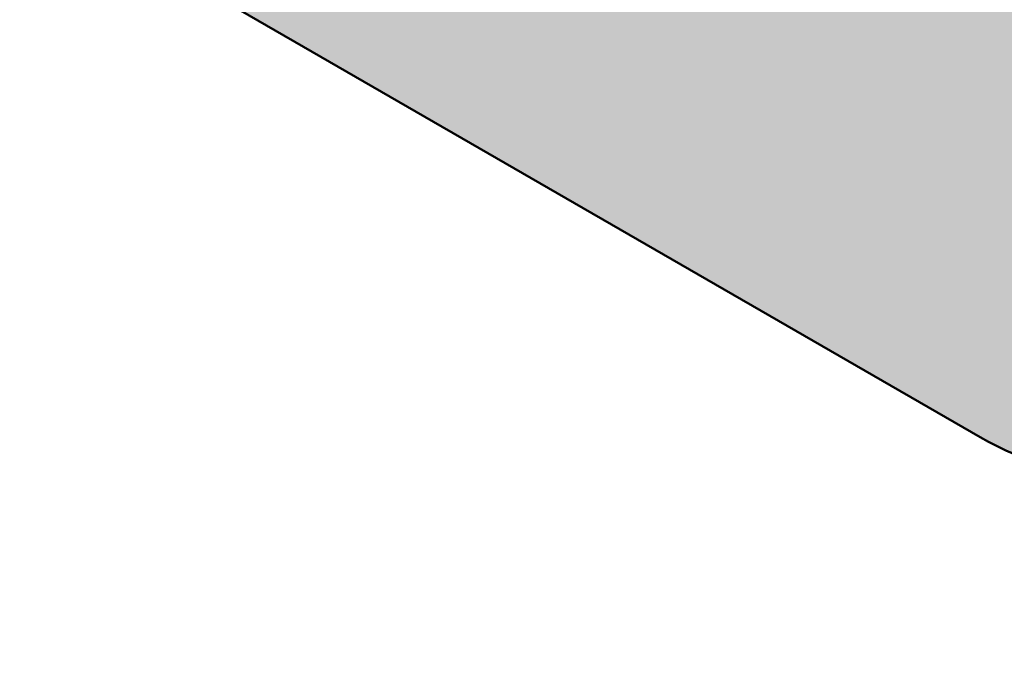
# Model space of a CAD drawing. Units: millimetres. Extents: x 0 to 2267, y 0 to 1823.
# Tile 22 of 256: x 1506 to 1590, y 1217 to 1271. Entities that reach past the tile are written whole.
import ezdxf

# ---------------------------------------------------------------- set-up
doc = ezdxf.new("R2010")
doc.units = ezdxf.units.MM
doc.header["$MEASUREMENT"] = 0
for name, color, linetype, lineweight in [('M-DIMS', 2, 'Continuous', 25), ('M-HATC', 252, 'Continuous', 18), ('M-OUTL', 7, 'Continuous', 50)]:
    doc.layers.add(name, color=color, linetype=linetype, lineweight=lineweight)
doc.styles.get("Standard").update_dxf_attribs({"font": 'arial.ttf'})
doc.dimstyles.get("Standard").update_dxf_attribs({"dimtxt": 7, "dimasz": 4, "dimexe": 0.18, "dimexo": 0.0625, "dimgap": 0.09, "dimtad": 0, "dimdec": 0, "dimzin": 0, "dimdsep": 46, "dimtxsty": 'Standard', "dimcen": 0.09, "dimadec": 0, "dimazin": 0, "dimtfac": 1, "dimtdec": 0, "dimtofl": 0, "dimtmove": 0, "dimatfit": 3, "dimfxl": 1, "dimtolj": 1, "dimtzin": 0, "dimarcsym": 0})

# ---------------------------------------------------------------- blocks, each defined once
blk = doc.blocks.new('*D19')
at = {"layer": 'Defpoints', "color": 0, "transparency": 16777216}
for p in [(1605.34, 1483.304), (1445.529, 1333.885)]:
    blk.add_point(p, dxfattribs=at)
at = {"layer": 'M-DIMS', "color": 0, "lineweight": -2, "transparency": 16777216}
for p, q in [((1605.25, 1483.304), (1605.43, 1483.304)), ((1605.34, 1483.214), (1605.34, 1483.394)), ((1366.324, 1259.831), (1442.607, 1331.153))]:
    blk.add_line(p, q, dxfattribs=at)
at = {"layer": 'M-DIMS', "color": 0, "transparency": 16777216}
blk.add_solid([(1442.152, 1331.64), (1443.063, 1330.666), (1445.529, 1333.885)], dxfattribs=at)
at = {"layer": 'M-DIMS', "color": 0, "transparency": 16777216, "insert": (1349.643, 1244.233), "char_height": 7, "attachment_point": 5, "rotation": 43.07533}
blk.add_mtext('\\A1;2X R218.8', dxfattribs=at)

msp = doc.modelspace()

# ---------------------------------------------------------------- hatches: boundary and pattern name
at = {"layer": 'M-HATC'}
h = msp.add_hatch(color=256, dxfattribs=at)
h.dxf.hatch_style = 1
h.paths.add_polyline_path([(2065.771, 1618.062, 0.236068), (2055.771, 1638.062), (1381.087, 1638.062, 0.236068), (1371.087, 1618.062), (1371.087, 1603.062), (2055.771, 1603.062), (2065.771, 1603.062)])
h.paths.add_polyline_path([(2062.772, 1550.296), (2062.772, 1560.296), (1374.086, 1560.296), (1374.086, 1550.296), (1374.086, 1540.296), (1384.086, 1540.296), (1389.086, 1540.296), (2062.772, 1540.296)])
h.paths.add_polyline_path([(1930.929, 1282.766), (1505.929, 1282.766), (1587.628, 1235.597, 0.131652), (1600.128, 1232.247), (1836.73, 1232.247, 0.131652), (1849.23, 1235.597)])
h.paths.add_polyline_path([(1930.929, 1117.417), (1905.929, 1117.417), (1505.929, 1117.417), (1505.929, 1077.417), (1930.929, 1077.417)])
h = msp.add_hatch(color=256, dxfattribs=at)
h.dxf.hatch_style = 1
h.paths.add_polyline_path([(2055.771, 1603.062), (1381.087, 1603.062), (1381.087, 1598.062), (2055.771, 1598.062)])
h.paths.add_polyline_path([(2055.771, 1598.062), (1381.087, 1598.062), (1381.087, 1593.062), (2055.771, 1593.062)])
h.paths.add_polyline_path([(2051.307, 1536.761), (1385.55, 1536.761), (1385.55, 1526.761), (1387.55, 1526.761), (1388.537, 1525.053), (1385.332, 1521.233), (1385.332, 1521.223), (2050.254, 1522.749), (2048.321, 1525.053), (2049.307, 1526.761), (2051.307, 1526.761)])
edge = h.paths.add_edge_path()
edge.add_arc((1847.535, 1379.149), 135, 222.60306, 222.89085, ccw=False)
edge.add_line((1748.166, 1287.766), (1683.092, 1287.766))
edge.add_arc((1583.724, 1379.149), 135, 317.10915, 317.39694, ccw=False)
edge.add_arc((1678.969, 1290.671), 5, 222.89085, 317.10915, ccw=False)
edge.add_arc((1774.213, 1379.149), 135, 222.60306, 222.89085, ccw=False)
edge.add_line((1674.845, 1287.766), (1609.771, 1287.766))
edge.add_arc((1510.403, 1379.149), 135, 317.10915, 317.39694, ccw=False)
edge.add_arc((1605.647, 1290.671), 5, 222.89085, 317.10915, ccw=False)
edge.add_arc((1700.892, 1379.149), 135, 222.60306, 222.89085, ccw=False)
edge.add_line((1601.524, 1287.766), (1536.45, 1287.766))
edge.add_arc((1437.081, 1379.149), 135, 317.10915, 317.39694, ccw=False)
edge.add_arc((1532.326, 1290.671), 5, 222.89085, 317.10915, ccw=False)
edge.add_arc((1627.571, 1379.149), 135, 222.60306, 222.89085, ccw=False)
edge.add_line((1528.203, 1287.766), (1505.929, 1287.766))
edge.add_spline(control_points=[(1505.929, 1287.766), (1504.262, 1287.766), (1504.262, 1282.766), (1505.929, 1282.766)], knot_values=[0, 0, 0, 0, 5, 5, 5, 5], degree=3, periodic=0)
edge.add_line((1505.929, 1282.766), (1930.929, 1282.766))
edge.add_spline(control_points=[(1930.929, 1282.766), (1932.596, 1282.766), (1932.596, 1287.766), (1930.929, 1287.766)], knot_values=[0, 0, 0, 0, 5, 5, 5, 5], degree=3, periodic=0)
edge.add_line((1930.929, 1287.766), (1903.056, 1287.766))
edge.add_arc((1803.688, 1379.149), 135, 317.10915, 317.39694, ccw=False)
edge.add_arc((1898.932, 1290.671), 5, 222.89085, 317.10915, ccw=False)
edge.add_arc((1994.177, 1379.149), 135, 222.60306, 222.89085, ccw=False)
edge.add_line((1894.809, 1287.766), (1829.735, 1287.766))
edge.add_arc((1730.366, 1379.149), 135, 317.10915, 317.39694, ccw=False)
edge.add_arc((1825.611, 1290.671), 5, 222.89085, 317.10915, ccw=False)
edge.add_arc((1920.856, 1379.149), 135, 222.60306, 222.89085, ccw=False)
edge.add_line((1821.487, 1287.766), (1756.413, 1287.766))
edge.add_arc((1657.045, 1379.149), 135, 317.10915, 317.39694, ccw=False)
edge.add_arc((1752.29, 1290.671), 5, 222.89085, 317.10915, ccw=False)
edge = h.paths.add_edge_path()
edge.add_spline(control_points=[(1843.429, 1227.247), (1845.096, 1227.247), (1845.096, 1232.247), (1843.429, 1232.247)], knot_values=[0, 0, 0, 0, 5, 5, 5, 5], degree=3, periodic=0)
edge.add_line((1843.429, 1232.247), (1593.429, 1232.247))
edge.add_spline(control_points=[(1593.429, 1232.247), (1591.762, 1232.247), (1591.762, 1227.247), (1593.429, 1227.247)], knot_values=[0, 0, 0, 0, 5, 5, 5, 5], degree=3, periodic=0)
edge.add_line((1593.429, 1227.247), (1843.429, 1227.247))
h.paths.add_polyline_path([(1905.929, 1127.417), (1530.929, 1127.417, 0.414214), (1520.929, 1117.417), (1530.929, 1117.417), (1915.929, 1117.417, 0.414214)])
edge = h.paths.add_edge_path()
edge.add_arc((1397.086, 1498.408), 12.73, 90.78215, 190.87871, ccw=False)
edge.add_line((1396.912, 1511.136), (1428.01, 1511.349))
edge.add_line((1428.01, 1511.349), (1433.01, 1511.349))
edge.add_line((1433.01, 1511.349), (1434.439, 1511.349))
edge.add_arc((1419.474, 1498.08), 20, 41.561, 74.08211)
edge.add_line((1424.959, 1517.314), (1399.935, 1517.256))
edge.add_spline(control_points=[(1399.931, 1517.256), (1399.884, 1517.213), (1399.833, 1517.169), (1399.777, 1517.124)], knot_values=[11.567499, 11.567499, 11.567499, 11.567499, 11.814249, 11.814249, 11.814249, 11.814249], degree=3, periodic=0)
edge.add_spline(control_points=[(1399.633, 1517.01), (1399.583, 1516.972), (1399.531, 1516.934), (1399.476, 1516.895)], knot_values=[11.167718, 11.167718, 11.167718, 11.167718, 11.365188, 11.365188, 11.365188, 11.365188], degree=3, periodic=0)
edge.add_spline(control_points=[(1399.34, 1516.8), (1399.151, 1516.672), (1398.938, 1516.538), (1398.704, 1516.399)], knot_values=[10.376405, 10.376405, 10.376405, 10.376405, 11.00994, 11.00994, 11.00994, 11.00994], degree=3, periodic=0)
edge.add_spline(control_points=[(1398.657, 1516.372), (1398.579, 1516.326), (1398.498, 1516.28), (1398.415, 1516.233)], knot_values=[10.125175, 10.125175, 10.125175, 10.125175, 10.334406, 10.334406, 10.334406, 10.334406], degree=3, periodic=0)
edge.add_spline(control_points=[(1398.264, 1516.149), (1398.196, 1516.111), (1398.126, 1516.073), (1398.055, 1516.035)], knot_values=[9.832246, 9.832246, 9.832246, 9.832246, 9.999658, 9.999658, 9.999658, 9.999658], degree=3, periodic=0)
edge.add_spline(control_points=[(1397.999, 1516.005), (1397.731, 1515.862), (1397.446, 1515.717), (1397.147, 1515.571)], knot_values=[9.161808, 9.161808, 9.161808, 9.161808, 9.787769, 9.787769, 9.787769, 9.787769], degree=3, periodic=0)
edge.add_spline(control_points=[(1397.147, 1515.571), (1396.842, 1515.423), (1396.522, 1515.274), (1396.191, 1515.126)], knot_values=[8.524455, 8.524455, 8.524455, 8.524455, 9.161808, 9.161808, 9.161808, 9.161808], degree=3, periodic=0)
edge.add_spline(control_points=[(1396.078, 1515.076), (1395.985, 1515.035), (1395.892, 1514.994), (1395.798, 1514.953)], knot_values=[8.275193, 8.275193, 8.275193, 8.275193, 8.451726, 8.451726, 8.451726, 8.451726], degree=3, periodic=0)
edge.add_spline(control_points=[(1395.602, 1514.869), (1395.5, 1514.826), (1395.397, 1514.782), (1395.293, 1514.739)], knot_values=[7.962917, 7.962917, 7.962917, 7.962917, 8.152764, 8.152764, 8.152764, 8.152764], degree=3, periodic=0)
edge.add_spline(control_points=[(1395.212, 1514.706), (1394.828, 1514.547), (1394.435, 1514.393), (1394.036, 1514.244)], knot_values=[7.21254, 7.21254, 7.21254, 7.21254, 7.913148, 7.913148, 7.913148, 7.913148], degree=3, periodic=0)
edge.add_spline(control_points=[(1394.036, 1514.244), (1393.708, 1514.121), (1393.375, 1514.003), (1393.043, 1513.889)], knot_values=[6.633733, 6.633733, 6.633733, 6.633733, 7.21254, 7.21254, 7.21254, 7.21254], degree=3, periodic=0)
edge.add_spline(control_points=[(1392.821, 1513.815), (1392.72, 1513.781), (1392.618, 1513.748), (1392.517, 1513.715)], knot_values=[6.328796, 6.328796, 6.328796, 6.328796, 6.505493, 6.505493, 6.505493, 6.505493], degree=3, periodic=0)
edge.add_spline(control_points=[(1392.517, 1513.715), (1392.319, 1513.652), (1392.121, 1513.59), (1391.924, 1513.531)], knot_values=[5.984605, 5.984605, 5.984605, 5.984605, 6.328796, 6.328796, 6.328796, 6.328796], degree=3, periodic=0)
edge.add_spline(control_points=[(1391.792, 1513.491), (1391.312, 1513.35), (1390.838, 1513.224), (1390.378, 1513.117)], knot_values=[5.066697, 5.066697, 5.066697, 5.066697, 5.907055, 5.907055, 5.907055, 5.907055], degree=3, periodic=0)
edge.add_spline(control_points=[(1390.378, 1513.117), (1390.18, 1513.071), (1389.984, 1513.028), (1389.791, 1512.99)], knot_values=[4.70367, 4.70367, 4.70367, 4.70367, 5.066695, 5.066695, 5.066695, 5.066695], degree=3, periodic=0)
edge.add_spline(control_points=[(1389.422, 1512.92), (1389.246, 1512.889), (1389.073, 1512.862), (1388.904, 1512.838)], knot_values=[4.130571, 4.130571, 4.130571, 4.130571, 4.469816, 4.469816, 4.469816, 4.469816], degree=3, periodic=0)
edge.add_spline(control_points=[(1388.904, 1512.838), (1388.591, 1512.795), (1388.291, 1512.764), (1388.007, 1512.749)], knot_values=[3.504031, 3.504031, 3.504031, 3.504031, 4.130571, 4.130571, 4.130571, 4.130571], degree=3, periodic=0)
edge.add_spline(control_points=[(1387.936, 1512.746), (1387.854, 1512.742), (1387.773, 1512.74), (1387.694, 1512.739)], knot_values=[3.268866, 3.268866, 3.268866, 3.268866, 3.451164, 3.451164, 3.451164, 3.451164], degree=3, periodic=0)
edge.add_spline(control_points=[(1387.335, 1512.744), (1387.208, 1512.75), (1387.085, 1512.76), (1386.967, 1512.774)], knot_values=[2.670686, 2.670686, 2.670686, 2.670686, 2.984, 2.984, 2.984, 2.984], degree=3, periodic=0)
edge.add_spline(control_points=[(1386.833, 1512.792), (1386.821, 1512.794), (1386.809, 1512.796), (1386.797, 1512.798)], knot_values=[2.516981, 2.516981, 2.516981, 2.516981, 2.549528, 2.549528, 2.549528, 2.549528], degree=3, periodic=0)
edge.add_spline(control_points=[(1386.453, 1512.873), (1386.426, 1512.881), (1386.399, 1512.889), (1386.373, 1512.897)], knot_values=[2.095869, 2.095869, 2.095869, 2.095869, 2.17941, 2.17941, 2.17941, 2.17941], degree=3, periodic=0)
edge.add_spline(control_points=[(1386.069, 1513.019), (1386.063, 1513.022), (1386.058, 1513.025), (1386.052, 1513.028)], knot_values=[1.72453, 1.72453, 1.72453, 1.72453, 1.745933, 1.745933, 1.745933, 1.745933], degree=3, periodic=0)
edge.add_arc((1399.474, 1498.08), 20, 131.82432, 180)
edge.add_arc((1630.334, 1505.548), 250.971, 181.70518, 236.42798)
edge.add_arc((1605.34, 1483.304), 218.782, 238.66083, 243.34961)
edge.add_arc((1647.091, 1510.359), 262.899, 183.12984, 237.85344, ccw=False)
h.paths.add_polyline_path([(1406.537, 1391.964, 0.149382), (1491.551, 1296.442, -0.129517)], flags=17)
edge = h.paths.add_edge_path()
edge.add_arc((2037.384, 1498.08), 20, 0, 48.26587)
edge.add_spline(control_points=[(2050.697, 1513.005), (2050.651, 1512.985), (2050.603, 1512.966), (2050.554, 1512.948)], knot_values=[1.835652, 1.835652, 1.835652, 1.835652, 2.000781, 2.000781, 2.000781, 2.000781], degree=3, periodic=0)
edge.add_spline(control_points=[(2050.462, 1512.917), (2050.479, 1512.922), (2050.496, 1512.928), (2050.513, 1512.934)], knot_values=[2.045477, 2.045477, 2.045477, 2.045477, 2.101389, 2.101389, 2.101389, 2.101389], degree=3, periodic=0)
edge.add_spline(control_points=[(2050.129, 1512.834), (2050.198, 1512.847), (2050.266, 1512.862), (2050.331, 1512.879)], knot_values=[2.237629, 2.237629, 2.237629, 2.237629, 2.435841, 2.435841, 2.435841, 2.435841], degree=3, periodic=0)
edge.add_spline(control_points=[(2050.095, 1512.828), (2050.106, 1512.83), (2050.118, 1512.832), (2050.129, 1512.834)], knot_values=[2.435841, 2.435841, 2.435841, 2.435841, 2.468321, 2.468321, 2.468321, 2.468321], degree=3, periodic=0)
edge.add_spline(control_points=[(2049.784, 1512.785), (2049.855, 1512.792), (2049.924, 1512.801), (2049.992, 1512.811)], knot_values=[2.563852, 2.563852, 2.563852, 2.563852, 2.748541, 2.748541, 2.748541, 2.748541], degree=3, periodic=0)
edge.add_spline(control_points=[(2049.405, 1512.762), (2049.536, 1512.765), (2049.663, 1512.773), (2049.784, 1512.785)], knot_values=[2.748541, 2.748541, 2.748541, 2.748541, 3.064882, 3.064882, 3.064882, 3.064882], degree=3, periodic=0)
edge.add_spline(control_points=[(2049.17, 1512.76), (2049.234, 1512.759), (2049.297, 1512.759), (2049.358, 1512.761)], knot_values=[3.102309, 3.102309, 3.102309, 3.102309, 3.2503, 3.2503, 3.2503, 3.2503], degree=3, periodic=0)
edge.add_spline(control_points=[(2048.857, 1512.769), (2048.964, 1512.764), (2049.068, 1512.761), (2049.17, 1512.76)], knot_values=[3.2503, 3.2503, 3.2503, 3.2503, 3.486069, 3.486069, 3.486069, 3.486069], degree=3, periodic=0)
edge.add_spline(control_points=[(2048.692, 1512.779), (2048.373, 1512.801), (2048.035, 1512.841), (2047.682, 1512.897)], knot_values=[3.606429, 3.606429, 3.606429, 3.606429, 4.2989, 4.2989, 4.2989, 4.2989], degree=3, periodic=0)
edge.add_spline(control_points=[(2047.682, 1512.897), (2047.546, 1512.919), (2047.408, 1512.942), (2047.268, 1512.969)], knot_values=[4.2989, 4.2989, 4.2989, 4.2989, 4.565769, 4.565769, 4.565769, 4.565769], degree=3, periodic=0)
edge.add_spline(control_points=[(2047.268, 1512.969), (2047.145, 1512.991), (2047.021, 1513.016), (2046.895, 1513.042)], knot_values=[4.565769, 4.565769, 4.565769, 4.565769, 4.799971, 4.799971, 4.799971, 4.799971], degree=3, periodic=0)
edge.add_spline(control_points=[(2046.895, 1513.042), (2046.529, 1513.119), (2046.151, 1513.209), (2045.768, 1513.311)], knot_values=[4.799971, 4.799971, 4.799971, 4.799971, 5.483718, 5.483718, 5.483718, 5.483718], degree=3, periodic=0)
edge.add_spline(control_points=[(2045.768, 1513.311), (2045.372, 1513.415), (2044.97, 1513.532), (2044.566, 1513.659)], knot_values=[5.483718, 5.483718, 5.483718, 5.483718, 6.187866, 6.187866, 6.187866, 6.187866], degree=3, periodic=0)
edge.add_spline(control_points=[(2044.566, 1513.659), (2044.415, 1513.706), (2044.263, 1513.755), (2044.112, 1513.805)], knot_values=[6.187866, 6.187866, 6.187866, 6.187866, 6.451551, 6.451551, 6.451551, 6.451551], degree=3, periodic=0)
edge.add_spline(control_points=[(2044.112, 1513.805), (2043.997, 1513.843), (2043.882, 1513.881), (2043.767, 1513.92)], knot_values=[6.451551, 6.451551, 6.451551, 6.451551, 6.651434, 6.651434, 6.651434, 6.651434], degree=3, periodic=0)
edge.add_spline(control_points=[(2043.767, 1513.92), (2043.372, 1514.055), (2042.977, 1514.198), (2042.589, 1514.346)], knot_values=[6.651434, 6.651434, 6.651434, 6.651434, 7.338879, 7.338879, 7.338879, 7.338879], degree=3, periodic=0)
edge.add_spline(control_points=[(2042.589, 1514.346), (2042.164, 1514.507), (2041.746, 1514.675), (2041.341, 1514.846)], knot_values=[7.338879, 7.338879, 7.338879, 7.338879, 8.089209, 8.089209, 8.089209, 8.089209], degree=3, periodic=0)
edge.add_spline(control_points=[(2041.341, 1514.846), (2041.103, 1514.946), (2040.869, 1515.048), (2040.64, 1515.15)], knot_values=[8.089209, 8.089209, 8.089209, 8.089209, 8.529587, 8.529587, 8.529587, 8.529587], degree=3, periodic=0)
edge.add_spline(control_points=[(2040.51, 1515.209), (2040.082, 1515.402), (2039.675, 1515.597), (2039.295, 1515.789)], knot_values=[8.613818, 8.613818, 8.613818, 8.613818, 9.44571, 9.44571, 9.44571, 9.44571], degree=3, periodic=0)
edge.add_spline(control_points=[(2039.295, 1515.789), (2039.062, 1515.907), (2038.839, 1516.025), (2038.629, 1516.14)], knot_values=[9.44571, 9.44571, 9.44571, 9.44571, 9.956404, 9.956404, 9.956404, 9.956404], degree=3, periodic=0)
edge.add_spline(control_points=[(2038.629, 1516.14), (2038.519, 1516.2), (2038.412, 1516.26), (2038.309, 1516.319)], knot_values=[9.956404, 9.956404, 9.956404, 9.956404, 10.223542, 10.223542, 10.223542, 10.223542], degree=3, periodic=0)
edge.add_spline(control_points=[(2038.309, 1516.319), (2038.214, 1516.374), (2038.122, 1516.428), (2038.033, 1516.481)], knot_values=[10.223542, 10.223542, 10.223542, 10.223542, 10.47051, 10.47051, 10.47051, 10.47051], degree=3, periodic=0)
edge.add_spline(control_points=[(2038.033, 1516.481), (2037.786, 1516.63), (2037.564, 1516.773), (2037.372, 1516.909)], knot_values=[10.47051, 10.47051, 10.47051, 10.47051, 11.15767, 11.15767, 11.15767, 11.15767], degree=3, periodic=0)
edge.add_spline(control_points=[(2037.372, 1516.909), (2037.279, 1516.975), (2037.193, 1517.04), (2037.114, 1517.102)], knot_values=[11.15767, 11.15767, 11.15767, 11.15767, 11.49227, 11.49227, 11.49227, 11.49227], degree=3, periodic=0)
edge.add_spline(control_points=[(2036.856, 1517.326), (2036.915, 1517.269), (2036.981, 1517.21), (2037.056, 1517.149)], knot_values=[11.577341, 11.577341, 11.577341, 11.577341, 11.91035, 11.91035, 11.91035, 11.91035], degree=3, periodic=0)
edge.add_spline(control_points=[(2036.807, 1517.375), (2036.823, 1517.359), (2036.839, 1517.342), (2036.856, 1517.326)], knot_values=[11.91035, 11.91035, 11.91035, 11.91035, 12.007402, 12.007402, 12.007402, 12.007402], degree=3, periodic=0)
edge.add_spline(control_points=[(2036.702, 1517.494), (2036.71, 1517.483), (2036.72, 1517.472), (2036.729, 1517.461)], knot_values=[12.184155, 12.184155, 12.184155, 12.184155, 12.255409, 12.255409, 12.255409, 12.255409], degree=3, periodic=0)
edge.add_spline(control_points=[(2036.616, 1517.621), (2036.62, 1517.613), (2036.624, 1517.606), (2036.629, 1517.598)], knot_values=[12.487913, 12.487913, 12.487913, 12.487913, 12.541035, 12.541035, 12.541035, 12.541035], degree=3, periodic=0)
edge.add_spline(control_points=[(2036.563, 1517.786), (2036.564, 1517.779), (2036.564, 1517.773), (2036.565, 1517.766)], knot_values=[12.911761, 12.911761, 12.911761, 12.911761, 12.968286, 12.968286, 12.968286, 12.968286], degree=3, periodic=0)
edge.add_spline(control_points=[(2036.617, 1517.93), (2036.612, 1517.926), (2036.609, 1517.921), (2036.605, 1517.916)], knot_values=[13.382527, 13.382527, 13.382527, 13.382527, 13.433791, 13.433791, 13.433791, 13.433791], degree=3, periodic=0)
edge.add_spline(control_points=[(2036.749, 1518.017), (2036.736, 1518.012), (2036.724, 1518.006), (2036.712, 1518)], knot_values=[13.726299, 13.726299, 13.726299, 13.726299, 13.809928, 13.809928, 13.809928, 13.809928], degree=3, periodic=0)
edge.add_spline(control_points=[(2036.86, 1518.053), (2036.839, 1518.047), (2036.818, 1518.042), (2036.799, 1518.035)], knot_values=[13.910887, 13.910887, 13.910887, 13.910887, 14.02153, 14.02153, 14.02153, 14.02153], degree=3, periodic=0)
edge.add_line((2036.964, 1518.08), (2032.384, 1518.08))
edge.add_line((2032.384, 1518.08), (2027.384, 1518.08))
edge.add_line((2027.384, 1518.08), (2022.384, 1518.08))
edge.add_line((2022.384, 1518.08), (2017.384, 1518.08))
edge.add_arc((2017.384, 1498.08), 20, 90, 138.439)
edge.add_line((2002.419, 1511.349), (2003.848, 1511.349))
edge.add_line((2003.848, 1511.349), (2008.848, 1511.349))
edge.add_line((2008.848, 1511.349), (2039.772, 1511.138))
edge.add_arc((2039.772, 1498.408), 12.73, -10.87871, 90, ccw=False)
edge.add_arc((1789.767, 1510.359), 262.899, 302.14656, 356.87016, ccw=False)
edge.add_arc((1831.518, 1483.304), 218.782, 296.65039, 301.33917)
edge.add_arc((1806.524, 1505.548), 250.971, 303.57202, 358.29482)
h.paths.add_polyline_path([(2030.321, 1391.964, -0.129517), (1945.307, 1296.442, 0.149382)], flags=17)
edge = h.paths.add_edge_path()
edge.add_spline(control_points=[(2037.246, 1518.082), (2037.29, 1518.081), (2037.336, 1518.08), (2037.384, 1518.08)], knot_values=[0.000012, 0.000012, 0.000012, 0.000012, 0.144754, 0.144754, 0.144754, 0.144754], degree=3, periodic=0)
edge.add_line((2037.336, 1518.08), (2037.01, 1518.08))
edge.add_spline(control_points=[(2037.01, 1518.08), (2036.982, 1518.077), (2036.956, 1518.073), (2036.931, 1518.068)], knot_values=[14.13465, 14.13465, 14.13465, 14.13465, 14.247197, 14.247197, 14.247197, 14.247197], degree=3, periodic=0)
edge.add_spline(control_points=[(2036.931, 1518.068), (2036.928, 1518.067), (2036.924, 1518.067), (2036.921, 1518.066)], knot_values=[14.118315, 14.118315, 14.118315, 14.118315, 14.13465, 14.13465, 14.13465, 14.13465], degree=3, periodic=0)
edge.add_spline(control_points=[(2036.921, 1518.066), (2036.912, 1518.064), (2036.903, 1518.063), (2036.895, 1518.061)], knot_values=[14.078086, 14.078086, 14.078086, 14.078086, 14.118315, 14.118315, 14.118315, 14.118315], degree=3, periodic=0)
edge.add_spline(control_points=[(2036.895, 1518.061), (2036.883, 1518.058), (2036.872, 1518.056), (2036.86, 1518.053)], knot_values=[14.02153, 14.02153, 14.02153, 14.02153, 14.078086, 14.078086, 14.078086, 14.078086], degree=3, periodic=0)
edge.add_spline(control_points=[(2036.86, 1518.053), (2036.839, 1518.047), (2036.818, 1518.042), (2036.799, 1518.035)], knot_values=[13.910887, 13.910887, 13.910887, 13.910887, 14.02153, 14.02153, 14.02153, 14.02153], degree=3, periodic=0)
edge.add_spline(control_points=[(2036.799, 1518.035), (2036.798, 1518.035), (2036.797, 1518.035), (2036.797, 1518.035)], knot_values=[13.906906, 13.906906, 13.906906, 13.906906, 13.910887, 13.910887, 13.910887, 13.910887], degree=3, periodic=0)
edge.add_spline(control_points=[(2036.797, 1518.035), (2036.788, 1518.032), (2036.78, 1518.029), (2036.772, 1518.026)], knot_values=[13.857826, 13.857826, 13.857826, 13.857826, 13.906906, 13.906906, 13.906906, 13.906906], degree=3, periodic=0)
edge.add_spline(control_points=[(2036.772, 1518.026), (2036.764, 1518.023), (2036.756, 1518.02), (2036.749, 1518.017)], knot_values=[13.809928, 13.809928, 13.809928, 13.809928, 13.857826, 13.857826, 13.857826, 13.857826], degree=3, periodic=0)
edge.add_spline(control_points=[(2036.749, 1518.017), (2036.736, 1518.012), (2036.724, 1518.006), (2036.712, 1518)], knot_values=[13.726299, 13.726299, 13.726299, 13.726299, 13.809928, 13.809928, 13.809928, 13.809928], degree=3, periodic=0)
edge.add_spline(control_points=[(2036.712, 1518), (2036.712, 1518), (2036.712, 1518), (2036.711, 1518)], knot_values=[13.723993, 13.723993, 13.723993, 13.723993, 13.726299, 13.726299, 13.726299, 13.726299], degree=3, periodic=0)
edge.add_spline(control_points=[(2036.711, 1518), (2036.706, 1517.997), (2036.701, 1517.994), (2036.696, 1517.992)], knot_values=[13.686536, 13.686536, 13.686536, 13.686536, 13.723993, 13.723993, 13.723993, 13.723993], degree=3, periodic=0)
edge.add_spline(control_points=[(2036.696, 1517.992), (2036.692, 1517.989), (2036.687, 1517.987), (2036.683, 1517.984)], knot_values=[13.651251, 13.651251, 13.651251, 13.651251, 13.686536, 13.686536, 13.686536, 13.686536], degree=3, periodic=0)
edge.add_spline(control_points=[(2036.683, 1517.984), (2036.676, 1517.98), (2036.67, 1517.976), (2036.664, 1517.971)], knot_values=[13.596804, 13.596804, 13.596804, 13.596804, 13.651251, 13.651251, 13.651251, 13.651251], degree=3, periodic=0)
edge.add_spline(control_points=[(2036.664, 1517.971), (2036.664, 1517.971), (2036.663, 1517.971), (2036.663, 1517.971)], knot_values=[13.593956, 13.593956, 13.593956, 13.593956, 13.596804, 13.596804, 13.596804, 13.596804], degree=3, periodic=0)
edge.add_spline(control_points=[(2036.663, 1517.971), (2036.66, 1517.969), (2036.658, 1517.967), (2036.655, 1517.965)], knot_values=[13.570322, 13.570322, 13.570322, 13.570322, 13.593956, 13.593956, 13.593956, 13.593956], degree=3, periodic=0)
edge.add_spline(control_points=[(2036.655, 1517.965), (2036.653, 1517.963), (2036.65, 1517.961), (2036.647, 1517.959)], knot_values=[13.545477, 13.545477, 13.545477, 13.545477, 13.570322, 13.570322, 13.570322, 13.570322], degree=3, periodic=0)
edge.add_spline(control_points=[(2036.647, 1517.959), (2036.647, 1517.959), (2036.647, 1517.959), (2036.647, 1517.959)], knot_values=[13.543931, 13.543931, 13.543931, 13.543931, 13.545477, 13.545477, 13.545477, 13.545477], degree=3, periodic=0)
edge.add_spline(control_points=[(2036.647, 1517.959), (2036.641, 1517.954), (2036.636, 1517.949), (2036.631, 1517.945)], knot_values=[13.488237, 13.488237, 13.488237, 13.488237, 13.543931, 13.543931, 13.543931, 13.543931], degree=3, periodic=0)
edge.add_spline(control_points=[(2036.631, 1517.945), (2036.628, 1517.942), (2036.626, 1517.94), (2036.623, 1517.937)], knot_values=[13.460307, 13.460307, 13.460307, 13.460307, 13.488237, 13.488237, 13.488237, 13.488237], degree=3, periodic=0)
edge.add_spline(control_points=[(2036.623, 1517.937), (2036.622, 1517.936), (2036.62, 1517.934), (2036.618, 1517.932)], knot_values=[13.439712, 13.439712, 13.439712, 13.439712, 13.460307, 13.460307, 13.460307, 13.460307], degree=3, periodic=0)
edge.add_spline(control_points=[(2036.618, 1517.932), (2036.618, 1517.931), (2036.617, 1517.931), (2036.617, 1517.93)], knot_values=[13.433791, 13.433791, 13.433791, 13.433791, 13.439712, 13.439712, 13.439712, 13.439712], degree=3, periodic=0)
edge.add_spline(control_points=[(2036.617, 1517.93), (2036.612, 1517.926), (2036.609, 1517.921), (2036.605, 1517.916)], knot_values=[13.382527, 13.382527, 13.382527, 13.382527, 13.433791, 13.433791, 13.433791, 13.433791], degree=3, periodic=0)
edge.add_spline(control_points=[(2036.605, 1517.916), (2036.603, 1517.913), (2036.6, 1517.91), (2036.598, 1517.907)], knot_values=[13.350017, 13.350017, 13.350017, 13.350017, 13.382527, 13.382527, 13.382527, 13.382527], degree=3, periodic=0)
edge.add_spline(control_points=[(2036.598, 1517.907), (2036.597, 1517.906), (2036.596, 1517.904), (2036.595, 1517.903)], knot_values=[13.333922, 13.333922, 13.333922, 13.333922, 13.350017, 13.350017, 13.350017, 13.350017], degree=3, periodic=0)
edge.add_spline(control_points=[(2036.595, 1517.903), (2036.595, 1517.902), (2036.594, 1517.901), (2036.593, 1517.9)], knot_values=[13.323828, 13.323828, 13.323828, 13.323828, 13.333922, 13.333922, 13.333922, 13.333922], degree=3, periodic=0)
edge.add_spline(control_points=[(2036.593, 1517.9), (2036.59, 1517.895), (2036.588, 1517.891), (2036.585, 1517.886)], knot_values=[13.277545, 13.277545, 13.277545, 13.277545, 13.323828, 13.323828, 13.323828, 13.323828], degree=3, periodic=0)
edge.add_spline(control_points=[(2036.585, 1517.886), (2036.584, 1517.883), (2036.582, 1517.879), (2036.58, 1517.875)], knot_values=[13.240119, 13.240119, 13.240119, 13.240119, 13.277545, 13.277545, 13.277545, 13.277545], degree=3, periodic=0)
edge.add_spline(control_points=[(2036.58, 1517.875), (2036.58, 1517.874), (2036.579, 1517.873), (2036.578, 1517.872)], knot_values=[13.228211, 13.228211, 13.228211, 13.228211, 13.240119, 13.240119, 13.240119, 13.240119], degree=3, periodic=0)
edge.add_spline(control_points=[(2036.578, 1517.872), (2036.578, 1517.87), (2036.577, 1517.869), (2036.577, 1517.868)], knot_values=[13.215717, 13.215717, 13.215717, 13.215717, 13.228211, 13.228211, 13.228211, 13.228211], degree=3, periodic=0)
edge.add_spline(control_points=[(2036.577, 1517.868), (2036.575, 1517.864), (2036.574, 1517.86), (2036.573, 1517.857)], knot_values=[13.179847, 13.179847, 13.179847, 13.179847, 13.215717, 13.215717, 13.215717, 13.215717], degree=3, periodic=0)
edge.add_spline(control_points=[(2036.573, 1517.857), (2036.571, 1517.851), (2036.57, 1517.846), (2036.569, 1517.841)], knot_values=[13.132017, 13.132017, 13.132017, 13.132017, 13.179847, 13.179847, 13.179847, 13.179847], degree=3, periodic=0)
edge.add_spline(control_points=[(2036.569, 1517.841), (2036.568, 1517.84), (2036.568, 1517.839), (2036.568, 1517.838)], knot_values=[13.122482, 13.122482, 13.122482, 13.122482, 13.132017, 13.132017, 13.132017, 13.132017], degree=3, periodic=0)
edge.add_spline(control_points=[(2036.568, 1517.838), (2036.568, 1517.836), (2036.567, 1517.835), (2036.567, 1517.833)], knot_values=[13.105592, 13.105592, 13.105592, 13.105592, 13.122482, 13.122482, 13.122482, 13.122482], degree=3, periodic=0)
edge.add_spline(control_points=[(2036.567, 1517.833), (2036.566, 1517.829), (2036.566, 1517.826), (2036.565, 1517.822)], knot_values=[13.074063, 13.074063, 13.074063, 13.074063, 13.105592, 13.105592, 13.105592, 13.105592], degree=3, periodic=0)
edge.add_spline(control_points=[(2036.565, 1517.822), (2036.565, 1517.822), (2036.565, 1517.822), (2036.565, 1517.822)], knot_values=[13.074043, 13.074043, 13.074043, 13.074043, 13.074063, 13.074063, 13.074063, 13.074063], degree=3, periodic=0)
edge.add_spline(control_points=[(2036.565, 1517.822), (2036.564, 1517.816), (2036.564, 1517.811), (2036.564, 1517.805)], knot_values=[13.021884, 13.021884, 13.021884, 13.021884, 13.074043, 13.074043, 13.074043, 13.074043], degree=3, periodic=0)
edge.add_spline(control_points=[(2036.564, 1517.805), (2036.564, 1517.804), (2036.564, 1517.803), (2036.564, 1517.803)], knot_values=[13.01674, 13.01674, 13.01674, 13.01674, 13.021884, 13.021884, 13.021884, 13.021884], degree=3, periodic=0)
edge.add_spline(control_points=[(2036.564, 1517.803), (2036.563, 1517.801), (2036.563, 1517.798), (2036.563, 1517.796)], knot_values=[12.996438, 12.996438, 12.996438, 12.996438, 13.01674, 13.01674, 13.01674, 13.01674], degree=3, periodic=0)
edge.add_spline(control_points=[(2036.563, 1517.796), (2036.563, 1517.793), (2036.563, 1517.789), (2036.563, 1517.786)], knot_values=[12.968286, 12.968286, 12.968286, 12.968286, 12.996438, 12.996438, 12.996438, 12.996438], degree=3, periodic=0)
edge.add_spline(control_points=[(2036.563, 1517.786), (2036.564, 1517.779), (2036.564, 1517.773), (2036.565, 1517.766)], knot_values=[12.911761, 12.911761, 12.911761, 12.911761, 12.968286, 12.968286, 12.968286, 12.968286], degree=3, periodic=0)
edge.add_spline(control_points=[(2036.565, 1517.766), (2036.565, 1517.766), (2036.565, 1517.766), (2036.565, 1517.766)], knot_values=[12.911017, 12.911017, 12.911017, 12.911017, 12.911761, 12.911761, 12.911761, 12.911761], degree=3, periodic=0)
edge.add_spline(control_points=[(2036.565, 1517.766), (2036.565, 1517.762), (2036.566, 1517.759), (2036.566, 1517.756)], knot_values=[12.88528, 12.88528, 12.88528, 12.88528, 12.911017, 12.911017, 12.911017, 12.911017], degree=3, periodic=0)
edge.add_spline(control_points=[(2036.566, 1517.756), (2036.567, 1517.753), (2036.567, 1517.751), (2036.568, 1517.748)], knot_values=[12.862519, 12.862519, 12.862519, 12.862519, 12.88528, 12.88528, 12.88528, 12.88528], degree=3, periodic=0)
edge.add_spline(control_points=[(2036.568, 1517.748), (2036.568, 1517.747), (2036.568, 1517.747), (2036.568, 1517.746)], knot_values=[12.858885, 12.858885, 12.858885, 12.858885, 12.862519, 12.862519, 12.862519, 12.862519], degree=3, periodic=0)
edge.add_spline(control_points=[(2036.568, 1517.746), (2036.569, 1517.74), (2036.571, 1517.733), (2036.572, 1517.726)], knot_values=[12.8053, 12.8053, 12.8053, 12.8053, 12.858885, 12.858885, 12.858885, 12.858885], degree=3, periodic=0)
edge.add_spline(control_points=[(2036.572, 1517.726), (2036.573, 1517.723), (2036.574, 1517.719), (2036.576, 1517.715)], knot_values=[12.775176, 12.775176, 12.775176, 12.775176, 12.8053, 12.8053, 12.8053, 12.8053], degree=3, periodic=0)
edge.add_spline(control_points=[(2036.576, 1517.715), (2036.576, 1517.713), (2036.577, 1517.71), (2036.578, 1517.708)], knot_values=[12.756759, 12.756759, 12.756759, 12.756759, 12.775176, 12.775176, 12.775176, 12.775176], degree=3, periodic=0)
edge.add_spline(control_points=[(2036.578, 1517.708), (2036.578, 1517.707), (2036.578, 1517.706), (2036.579, 1517.705)], knot_values=[12.748742, 12.748742, 12.748742, 12.748742, 12.756759, 12.756759, 12.756759, 12.756759], degree=3, periodic=0)
edge.add_spline(control_points=[(2036.579, 1517.705), (2036.581, 1517.698), (2036.583, 1517.692), (2036.586, 1517.685)], knot_values=[12.69959, 12.69959, 12.69959, 12.69959, 12.748742, 12.748742, 12.748742, 12.748742], degree=3, periodic=0)
edge.add_spline(control_points=[(2036.586, 1517.685), (2036.588, 1517.68), (2036.59, 1517.675), (2036.592, 1517.669)], knot_values=[12.659038, 12.659038, 12.659038, 12.659038, 12.69959, 12.69959, 12.69959, 12.69959], degree=3, periodic=0)
edge.add_spline(control_points=[(2036.592, 1517.669), (2036.594, 1517.665), (2036.596, 1517.66), (2036.598, 1517.656)], knot_values=[12.626806, 12.626806, 12.626806, 12.626806, 12.659038, 12.659038, 12.659038, 12.659038], degree=3, periodic=0)
edge.add_spline(control_points=[(2036.598, 1517.656), (2036.598, 1517.655), (2036.599, 1517.654), (2036.599, 1517.653)], knot_values=[12.619394, 12.619394, 12.619394, 12.619394, 12.626806, 12.626806, 12.626806, 12.626806], degree=3, periodic=0)
edge.add_spline(control_points=[(2036.599, 1517.653), (2036.604, 1517.642), (2036.61, 1517.632), (2036.616, 1517.621)], knot_values=[12.541039, 12.541039, 12.541039, 12.541039, 12.619394, 12.619394, 12.619394, 12.619394], degree=3, periodic=0)
edge.add_spline(control_points=[(2036.616, 1517.621), (2036.616, 1517.621), (2036.616, 1517.621), (2036.616, 1517.621)], knot_values=[12.541035, 12.541035, 12.541035, 12.541035, 12.541039, 12.541039, 12.541039, 12.541039], degree=3, periodic=0)
edge.add_spline(control_points=[(2036.616, 1517.621), (2036.62, 1517.613), (2036.624, 1517.606), (2036.629, 1517.598)], knot_values=[12.487913, 12.487913, 12.487913, 12.487913, 12.541035, 12.541035, 12.541035, 12.541035], degree=3, periodic=0)
edge.add_spline(control_points=[(2036.629, 1517.598), (2036.633, 1517.592), (2036.637, 1517.585), (2036.641, 1517.579)], knot_values=[12.443982, 12.443982, 12.443982, 12.443982, 12.487913, 12.487913, 12.487913, 12.487913], degree=3, periodic=0)
edge.add_spline(control_points=[(2036.641, 1517.579), (2036.641, 1517.578), (2036.642, 1517.576), (2036.643, 1517.575)], knot_values=[12.434996, 12.434996, 12.434996, 12.434996, 12.443982, 12.443982, 12.443982, 12.443982], degree=3, periodic=0)
edge.add_spline(control_points=[(2036.643, 1517.575), (2036.653, 1517.56), (2036.664, 1517.544), (2036.676, 1517.528)], knot_values=[12.329647, 12.329647, 12.329647, 12.329647, 12.434996, 12.434996, 12.434996, 12.434996], degree=3, periodic=0)
edge.add_spline(control_points=[(2036.676, 1517.528), (2036.684, 1517.517), (2036.693, 1517.505), (2036.702, 1517.494)], knot_values=[12.255409, 12.255409, 12.255409, 12.255409, 12.329647, 12.329647, 12.329647, 12.329647], degree=3, periodic=0)
edge.add_spline(control_points=[(2036.702, 1517.494), (2036.71, 1517.483), (2036.72, 1517.472), (2036.729, 1517.461)], knot_values=[12.184155, 12.184155, 12.184155, 12.184155, 12.255409, 12.255409, 12.255409, 12.255409], degree=3, periodic=0)
edge.add_spline(control_points=[(2036.729, 1517.461), (2036.744, 1517.444), (2036.759, 1517.426), (2036.775, 1517.409)], knot_values=[12.075961, 12.075961, 12.075961, 12.075961, 12.184155, 12.184155, 12.184155, 12.184155], degree=3, periodic=0)
edge.add_spline(control_points=[(2036.775, 1517.409), (2036.776, 1517.407), (2036.777, 1517.406), (2036.778, 1517.405)], knot_values=[12.069502, 12.069502, 12.069502, 12.069502, 12.075961, 12.075961, 12.075961, 12.075961], degree=3, periodic=0)
edge.add_spline(control_points=[(2036.778, 1517.405), (2036.788, 1517.395), (2036.797, 1517.385), (2036.807, 1517.375)], knot_values=[12.007402, 12.007402, 12.007402, 12.007402, 12.069502, 12.069502, 12.069502, 12.069502], degree=3, periodic=0)
edge.add_spline(control_points=[(2036.807, 1517.375), (2036.823, 1517.359), (2036.839, 1517.342), (2036.856, 1517.326)], knot_values=[11.91035, 11.91035, 11.91035, 11.91035, 12.007402, 12.007402, 12.007402, 12.007402], degree=3, periodic=0)
edge.add_spline(control_points=[(2036.856, 1517.326), (2036.915, 1517.269), (2036.981, 1517.21), (2037.056, 1517.149)], knot_values=[11.577341, 11.577341, 11.577341, 11.577341, 11.91035, 11.91035, 11.91035, 11.91035], degree=3, periodic=0)
edge.add_spline(control_points=[(2037.056, 1517.149), (2037.075, 1517.134), (2037.094, 1517.118), (2037.114, 1517.102)], knot_values=[11.49227, 11.49227, 11.49227, 11.49227, 11.577341, 11.577341, 11.577341, 11.577341], degree=3, periodic=0)
edge.add_spline(control_points=[(2037.114, 1517.102), (2037.193, 1517.04), (2037.279, 1516.975), (2037.372, 1516.909)], knot_values=[11.15767, 11.15767, 11.15767, 11.15767, 11.49227, 11.49227, 11.49227, 11.49227], degree=3, periodic=0)
edge.add_spline(control_points=[(2037.372, 1516.909), (2037.564, 1516.773), (2037.786, 1516.63), (2038.033, 1516.481)], knot_values=[10.47051, 10.47051, 10.47051, 10.47051, 11.15767, 11.15767, 11.15767, 11.15767], degree=3, periodic=0)
edge.add_spline(control_points=[(2038.033, 1516.481), (2038.122, 1516.428), (2038.214, 1516.374), (2038.309, 1516.319)], knot_values=[10.223542, 10.223542, 10.223542, 10.223542, 10.47051, 10.47051, 10.47051, 10.47051], degree=3, periodic=0)
edge.add_spline(control_points=[(2038.309, 1516.319), (2038.412, 1516.26), (2038.519, 1516.2), (2038.629, 1516.14)], knot_values=[9.956404, 9.956404, 9.956404, 9.956404, 10.223542, 10.223542, 10.223542, 10.223542], degree=3, periodic=0)
edge.add_spline(control_points=[(2038.629, 1516.14), (2038.839, 1516.025), (2039.062, 1515.907), (2039.295, 1515.789)], knot_values=[9.44571, 9.44571, 9.44571, 9.44571, 9.956404, 9.956404, 9.956404, 9.956404], degree=3, periodic=0)
edge.add_spline(control_points=[(2039.295, 1515.789), (2039.675, 1515.597), (2040.082, 1515.402), (2040.51, 1515.209)], knot_values=[8.613818, 8.613818, 8.613818, 8.613818, 9.44571, 9.44571, 9.44571, 9.44571], degree=3, periodic=0)
edge.add_spline(control_points=[(2040.51, 1515.209), (2040.553, 1515.189), (2040.597, 1515.17), (2040.64, 1515.15)], knot_values=[8.529587, 8.529587, 8.529587, 8.529587, 8.613818, 8.613818, 8.613818, 8.613818], degree=3, periodic=0)
edge.add_spline(control_points=[(2040.64, 1515.15), (2040.869, 1515.048), (2041.103, 1514.946), (2041.341, 1514.846)], knot_values=[8.089209, 8.089209, 8.089209, 8.089209, 8.529587, 8.529587, 8.529587, 8.529587], degree=3, periodic=0)
edge.add_spline(control_points=[(2041.341, 1514.846), (2041.746, 1514.675), (2042.164, 1514.507), (2042.589, 1514.346)], knot_values=[7.338879, 7.338879, 7.338879, 7.338879, 8.089209, 8.089209, 8.089209, 8.089209], degree=3, periodic=0)
edge.add_spline(control_points=[(2042.589, 1514.346), (2042.977, 1514.198), (2043.372, 1514.055), (2043.767, 1513.92)], knot_values=[6.651434, 6.651434, 6.651434, 6.651434, 7.338879, 7.338879, 7.338879, 7.338879], degree=3, periodic=0)
edge.add_spline(control_points=[(2043.767, 1513.92), (2043.882, 1513.881), (2043.997, 1513.843), (2044.112, 1513.805)], knot_values=[6.451551, 6.451551, 6.451551, 6.451551, 6.651434, 6.651434, 6.651434, 6.651434], degree=3, periodic=0)
edge.add_spline(control_points=[(2044.112, 1513.805), (2044.263, 1513.755), (2044.415, 1513.706), (2044.566, 1513.659)], knot_values=[6.187866, 6.187866, 6.187866, 6.187866, 6.451551, 6.451551, 6.451551, 6.451551], degree=3, periodic=0)
edge.add_spline(control_points=[(2044.566, 1513.659), (2044.97, 1513.532), (2045.372, 1513.415), (2045.768, 1513.311)], knot_values=[5.483718, 5.483718, 5.483718, 5.483718, 6.187866, 6.187866, 6.187866, 6.187866], degree=3, periodic=0)
edge.add_spline(control_points=[(2045.768, 1513.311), (2046.151, 1513.209), (2046.529, 1513.119), (2046.895, 1513.042)], knot_values=[4.799971, 4.799971, 4.799971, 4.799971, 5.483718, 5.483718, 5.483718, 5.483718], degree=3, periodic=0)
edge.add_spline(control_points=[(2046.895, 1513.042), (2047.021, 1513.016), (2047.145, 1512.991), (2047.268, 1512.969)], knot_values=[4.565769, 4.565769, 4.565769, 4.565769, 4.799971, 4.799971, 4.799971, 4.799971], degree=3, periodic=0)
edge.add_spline(control_points=[(2047.268, 1512.969), (2047.408, 1512.942), (2047.546, 1512.919), (2047.682, 1512.897)], knot_values=[4.2989, 4.2989, 4.2989, 4.2989, 4.565769, 4.565769, 4.565769, 4.565769], degree=3, periodic=0)
edge.add_spline(control_points=[(2047.682, 1512.897), (2048.035, 1512.841), (2048.373, 1512.801), (2048.692, 1512.779)], knot_values=[3.606429, 3.606429, 3.606429, 3.606429, 4.2989, 4.2989, 4.2989, 4.2989], degree=3, periodic=0)
edge.add_spline(control_points=[(2048.692, 1512.779), (2048.748, 1512.775), (2048.803, 1512.772), (2048.857, 1512.769)], knot_values=[3.486069, 3.486069, 3.486069, 3.486069, 3.606429, 3.606429, 3.606429, 3.606429], degree=3, periodic=0)
edge.add_spline(control_points=[(2048.857, 1512.769), (2048.964, 1512.764), (2049.068, 1512.761), (2049.17, 1512.76)], knot_values=[3.2503, 3.2503, 3.2503, 3.2503, 3.486069, 3.486069, 3.486069, 3.486069], degree=3, periodic=0)
edge.add_spline(control_points=[(2049.17, 1512.76), (2049.234, 1512.759), (2049.297, 1512.759), (2049.358, 1512.761)], knot_values=[3.102309, 3.102309, 3.102309, 3.102309, 3.2503, 3.2503, 3.2503, 3.2503], degree=3, periodic=0)
edge.add_spline(control_points=[(2049.358, 1512.761), (2049.374, 1512.761), (2049.39, 1512.761), (2049.405, 1512.762)], knot_values=[3.064882, 3.064882, 3.064882, 3.064882, 3.102309, 3.102309, 3.102309, 3.102309], degree=3, periodic=0)
edge.add_spline(control_points=[(2049.405, 1512.762), (2049.536, 1512.765), (2049.663, 1512.773), (2049.784, 1512.785)], knot_values=[2.748541, 2.748541, 2.748541, 2.748541, 3.064882, 3.064882, 3.064882, 3.064882], degree=3, periodic=0)
edge.add_spline(control_points=[(2049.784, 1512.785), (2049.855, 1512.792), (2049.924, 1512.801), (2049.992, 1512.811)], knot_values=[2.563852, 2.563852, 2.563852, 2.563852, 2.748541, 2.748541, 2.748541, 2.748541], degree=3, periodic=0)
edge.add_spline(control_points=[(2049.992, 1512.811), (2050.026, 1512.816), (2050.061, 1512.822), (2050.095, 1512.828)], knot_values=[2.468321, 2.468321, 2.468321, 2.468321, 2.563852, 2.563852, 2.563852, 2.563852], degree=3, periodic=0)
edge.add_spline(control_points=[(2050.095, 1512.828), (2050.106, 1512.83), (2050.118, 1512.832), (2050.129, 1512.834)], knot_values=[2.435841, 2.435841, 2.435841, 2.435841, 2.468321, 2.468321, 2.468321, 2.468321], degree=3, periodic=0)
edge.add_spline(control_points=[(2050.129, 1512.834), (2050.198, 1512.847), (2050.266, 1512.862), (2050.331, 1512.879)], knot_values=[2.237629, 2.237629, 2.237629, 2.237629, 2.435841, 2.435841, 2.435841, 2.435841], degree=3, periodic=0)
edge.add_spline(control_points=[(2050.331, 1512.879), (2050.375, 1512.891), (2050.419, 1512.903), (2050.462, 1512.917)], knot_values=[2.101389, 2.101389, 2.101389, 2.101389, 2.237629, 2.237629, 2.237629, 2.237629], degree=3, periodic=0)
edge.add_spline(control_points=[(2050.462, 1512.917), (2050.479, 1512.922), (2050.496, 1512.928), (2050.513, 1512.934)], knot_values=[2.045477, 2.045477, 2.045477, 2.045477, 2.101389, 2.101389, 2.101389, 2.101389], degree=3, periodic=0)
edge.add_spline(control_points=[(2050.513, 1512.934), (2050.527, 1512.938), (2050.54, 1512.943), (2050.554, 1512.948)], knot_values=[2.000781, 2.000781, 2.000781, 2.000781, 2.045477, 2.045477, 2.045477, 2.045477], degree=3, periodic=0)
edge.add_spline(control_points=[(2050.554, 1512.948), (2050.603, 1512.966), (2050.651, 1512.985), (2050.697, 1513.005)], knot_values=[1.835652, 1.835652, 1.835652, 1.835652, 2.000781, 2.000781, 2.000781, 2.000781], degree=3, periodic=0)
edge.add_arc((2037.384, 1498.08), 20, 48.26587, 90.12993)
edge = h.paths.add_edge_path(flags=16)
edge.add_spline(control_points=[(1386.139, 1512.986), (1388.92, 1511.739), (1398.039, 1515.519), (1399.931, 1517.256)], knot_values=[1.831046, 1.831046, 1.831046, 1.831046, 11.814249, 11.814249, 11.814249, 11.814249], degree=3, periodic=0)
edge.add_line((1399.931, 1517.256), (1393.743, 1517.242))
edge.add_arc((1399.474, 1498.08), 20, 106.6501, 131.8173)

# ---------------------------------------------------------------- linework, layer by layer
at = {"layer": 'M-OUTL'}
msp.add_line((1587.628, 1235.597), (1505.929, 1282.766), dxfattribs=at)
msp.add_arc((1600.128, 1257.247), 25, 240, 270, dxfattribs=at)

# ---------------------------------------------------------------- dimensions: what is measured, and where the dimension line sits
at = {"layer": 'M-DIMS'}
dim = msp.add_radius_dim(center=(1605.34, 1483.304), mpoint=(1445.529, 1333.885), text='2X <>', dimstyle='Standard', override={"dimdec": 1, "dimlfac": 1, "dimrnd": 0, "dimzin": 0, "dimdsep": 46, "dimlunit": 2}, dxfattribs=at)
dim.commit()
dim.dimension.update_dxf_attribs({"geometry": '*D19', "text_midpoint": (1349.643, 1244.233), "dimtype": 164})

doc.saveas('drawing.dxf')
